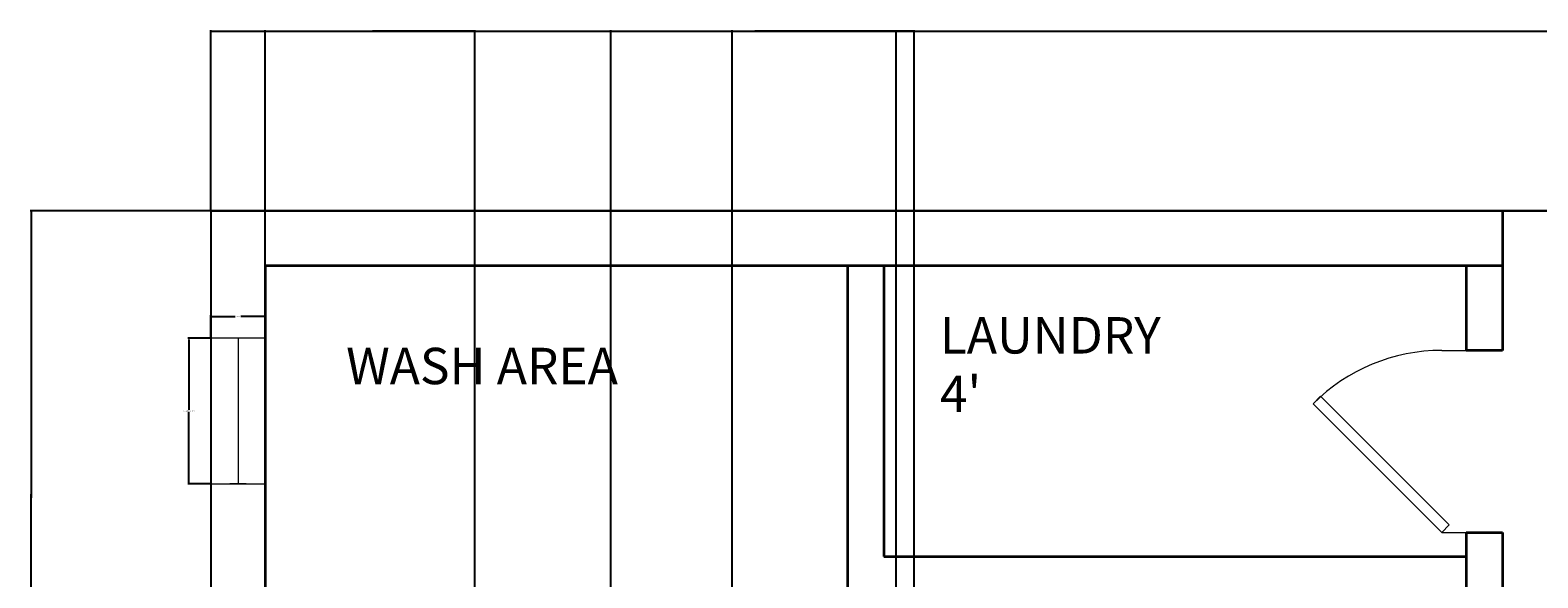
# Model space of a CAD drawing. Units: inches. Extents: x 450 to 1026, y 542 to 1190.
# Tile 9 of 11: x 450 to 698, y 1099 to 1190. Entities that reach past the tile are written whole.
import ezdxf

# ---------------------------------------------------------------- set-up
doc = ezdxf.new("R2010")
doc.units = ezdxf.units.IN
doc.header["$MEASUREMENT"] = 0
for name, color, linetype, lineweight in [('A-ANNO-DIMS', 2, 'Continuous', 18), ('A-AREA-IDEN', 7, 'Continuous', 18), ('A-DOOR', 4, 'Continuous', 18), ('A-GLAZ', 4, 'Continuous', 18), ('A-WALL', 7, 'Continuous', 35), ('C-PROP', 7, 'Continuous', 25)]:
    doc.layers.add(name, color=color, linetype=linetype, lineweight=lineweight)
doc.styles.get("Standard").update_dxf_attribs({"font": 'arial.ttf'})
doc.dimstyles.get("Standard").update_dxf_attribs({"dimtxt": 0.18, "dimasz": 0.18, "dimexe": 0.18, "dimexo": 0.0625, "dimgap": 0.09, "dimtad": 0, "dimtih": 1, "dimtoh": 1, "dimdec": 4, "dimzin": 0, "dimdsep": 46, "dimtxsty": 'Standard', "dimcen": 0.09, "dimadec": 0, "dimazin": 0, "dimtfac": 1, "dimtdec": 4, "dimtofl": 0, "dimtmove": 0, "dimatfit": 3, "dimfxl": 1, "dimtolj": 1, "dimtzin": 0, "dimarcsym": 0})

# ---------------------------------------------------------------- blocks, each defined once
blk = doc.blocks.new('*U4')
for p, q in [((0, 0), (0, -100)), ((750, 0), (750, -100))]:
    blk.add_line(p, q)
blk.add_lwpolyline([(0, 0), (530.3, 530.3), (561.3, 499.4), (30.9, -30.9)], close=True)
blk.add_arc((0, 0), 750, 0, 45)
blk = doc.blocks.new('*U3')
for p, q in [((0, 100), (0, 0)), ((900, 100), (900, 0)), ((0, 50), (900, 50))]:
    blk.add_line(p, q)
blk = doc.blocks.new('WIN-FRAME-24IN')
for p, q in [((9, 24), (0, 24)), ((0, 24), (0, 0)), ((0, 0), (9, 0))]:
    blk.add_line(p, q)
blk = doc.blocks.new('*D37')
at = {"layer": 'A-ANNO-DIMS', "color": 0, "lineweight": -2, "transparency": 16777216}
for p, q in [((479.59, 1138.94), (475.87, 1138.94)), ((476.05, 1138.76), (476.05, 1127.13)), ((476.05, 1115.12), (476.05, 1126.76)), ((479.59, 1114.94), (475.87, 1114.94))]:
    blk.add_line(p, q, dxfattribs=at)
at = {"layer": 'A-ANNO-DIMS', "color": 0, "transparency": 16777216}
for points in [[(476.02, 1138.76), (476.08, 1138.76), (476.05, 1138.94)], [(476.02, 1115.12), (476.08, 1115.12), (476.05, 1114.94)]]:
    blk.add_solid(points, dxfattribs=at)
at = {"layer": 'Defpoints', "color": 0, "transparency": 16777216}
for p in [(476.05, 1138.94), (479.65, 1138.94), (479.65, 1114.94)]:
    blk.add_point(p, dxfattribs=at)
at = {"layer": 'A-ANNO-DIMS', "color": 0, "transparency": 16777216, "insert": (476.05, 1126.94), "char_height": 0.18, "attachment_point": 5}
blk.add_mtext('\\A1;WINDOW 24 TYP.', dxfattribs=at)
blk = doc.blocks.new('*D38')
at = {"layer": 'A-ANNO-DIMS', "color": 0, "lineweight": -2, "transparency": 16777216}
for p, q in [((479.65, 1139.01), (479.65, 1142.72)), ((479.83, 1142.54), (483.69, 1142.54)), ((488.47, 1142.54), (484.61, 1142.54)), ((488.65, 1139.01), (488.65, 1142.72))]:
    blk.add_line(p, q, dxfattribs=at)
at = {"layer": 'A-ANNO-DIMS', "color": 0, "transparency": 16777216}
for points in [[(479.83, 1142.57), (479.83, 1142.51), (479.65, 1142.54)], [(488.47, 1142.57), (488.47, 1142.51), (488.65, 1142.54)]]:
    blk.add_solid(points, dxfattribs=at)
at = {"layer": 'Defpoints', "color": 0, "transparency": 16777216}
for p in [(488.65, 1142.54), (479.65, 1138.94), (488.65, 1138.94)]:
    blk.add_point(p, dxfattribs=at)
at = {"layer": 'A-ANNO-DIMS', "color": 0, "transparency": 16777216, "insert": (484.15, 1142.54), "char_height": 0.18, "attachment_point": 5}
blk.add_mtext('\\A1;9 TYP.', dxfattribs=at)
blk = doc.blocks.new('*D47')
at = {"layer": 'A-ANNO-DIMS', "color": 0, "lineweight": -2, "transparency": 16777216}
for p, q in [((479.65, 1160.01), (479.65, 1189.72)), ((479.83, 1189.54), (719.36, 1189.54)), ((959.47, 1189.54), (719.94, 1189.54)), ((959.65, 1065.01), (959.65, 1189.72))]:
    blk.add_line(p, q, dxfattribs=at)
at = {"layer": 'A-ANNO-DIMS', "color": 0, "transparency": 16777216}
for points in [[(479.83, 1189.57), (479.83, 1189.51), (479.65, 1189.54)], [(959.47, 1189.57), (959.47, 1189.51), (959.65, 1189.54)]]:
    blk.add_solid(points, dxfattribs=at)
at = {"layer": 'Defpoints', "color": 0, "transparency": 16777216}
for p in [(959.65, 1189.54), (479.65, 1159.94), (959.65, 1064.94)]:
    blk.add_point(p, dxfattribs=at)
at = {"layer": 'A-ANNO-DIMS', "color": 0, "transparency": 16777216, "insert": (719.65, 1189.54), "char_height": 0.18, "attachment_point": 5}
blk.add_mtext('\\A1;480', dxfattribs=at)
blk = doc.blocks.new('*D49')
at = {"layer": 'A-ANNO-DIMS', "color": 0, "lineweight": -2, "transparency": 16777216}
for p, q in [((479.59, 1159.94), (449.87, 1159.94)), ((450.05, 1159.76), (450.05, 1113.62)), ((450.05, 1067.12), (450.05, 1113.26)), ((479.59, 1066.94), (449.87, 1066.94))]:
    blk.add_line(p, q, dxfattribs=at)
at = {"layer": 'A-ANNO-DIMS', "color": 0, "transparency": 16777216}
for points in [[(450.02, 1159.76), (450.08, 1159.76), (450.05, 1159.94)], [(450.02, 1067.12), (450.08, 1067.12), (450.05, 1066.94)]]:
    blk.add_solid(points, dxfattribs=at)
at = {"layer": 'Defpoints', "color": 0, "transparency": 16777216}
for p in [(479.65, 1159.94), (450.05, 1066.94), (479.65, 1066.94)]:
    blk.add_point(p, dxfattribs=at)
at = {"layer": 'A-ANNO-DIMS', "color": 0, "transparency": 16777216, "insert": (450.05, 1113.44), "char_height": 0.18, "attachment_point": 5}
blk.add_mtext('\\A1;93', dxfattribs=at)
blk = doc.blocks.new('*D55')
at = {"layer": 'A-ANNO-DIMS', "color": 0, "lineweight": -2, "transparency": 16777216}
for p, q in [((995.59, 1159.94), (449.87, 1159.94)), ((450.05, 1159.76), (450.05, 1112.62)), ((450.05, 1065.12), (450.05, 1112.26)), ((959.59, 1064.94), (449.87, 1064.94))]:
    blk.add_line(p, q, dxfattribs=at)
at = {"layer": 'A-ANNO-DIMS', "color": 0, "transparency": 16777216}
for points in [[(450.02, 1159.76), (450.08, 1159.76), (450.05, 1159.94)], [(450.02, 1065.12), (450.08, 1065.12), (450.05, 1064.94)]]:
    blk.add_solid(points, dxfattribs=at)
at = {"layer": 'Defpoints', "color": 0, "transparency": 16777216}
for p in [(995.65, 1159.94), (450.05, 1064.94), (959.65, 1064.94)]:
    blk.add_point(p, dxfattribs=at)
at = {"layer": 'A-ANNO-DIMS', "color": 0, "transparency": 16777216, "insert": (450.05, 1112.44), "char_height": 0.18, "attachment_point": 5}
blk.add_mtext('\\A1;95', dxfattribs=at)
blk = doc.blocks.new('*D56')
at = {"layer": 'A-ANNO-DIMS', "color": 0, "lineweight": -2, "transparency": 16777216}
for p, q in [((488.65, 1150.88), (488.65, 542.16)), ((584.65, 1150.88), (584.65, 542.16)), ((488.83, 542.34), (536.43, 542.34)), ((584.47, 542.34), (536.87, 542.34))]:
    blk.add_line(p, q, dxfattribs=at)
at = {"layer": 'A-ANNO-DIMS', "color": 0, "transparency": 16777216}
for points in [[(488.83, 542.37), (488.83, 542.31), (488.65, 542.34)], [(584.47, 542.37), (584.47, 542.31), (584.65, 542.34)]]:
    blk.add_solid(points, dxfattribs=at)
at = {"layer": 'Defpoints', "color": 0, "transparency": 16777216}
for p in [(488.65, 1150.94), (584.65, 1150.94), (584.65, 542.34)]:
    blk.add_point(p, dxfattribs=at)
at = {"layer": 'A-ANNO-DIMS', "color": 0, "transparency": 16777216, "insert": (536.65, 542.34), "char_height": 0.18, "attachment_point": 5}
blk.add_mtext('\\A1;96', dxfattribs=at)
blk = doc.blocks.new('*D58')
at = {"layer": 'A-ANNO-DIMS', "color": 0, "lineweight": -2, "transparency": 16777216}
for p, q in [((545.65, 971.01), (545.65, 1189.72)), ((545.83, 1189.54), (568.93, 1189.54)), ((592.47, 1189.54), (569.37, 1189.54)), ((592.65, 977.01), (592.65, 1189.72))]:
    blk.add_line(p, q, dxfattribs=at)
at = {"layer": 'A-ANNO-DIMS', "color": 0, "transparency": 16777216}
for points in [[(545.83, 1189.57), (545.83, 1189.51), (545.65, 1189.54)], [(592.47, 1189.57), (592.47, 1189.51), (592.65, 1189.54)]]:
    blk.add_solid(points, dxfattribs=at)
at = {"layer": 'Defpoints', "color": 0, "transparency": 16777216}
for p in [(592.65, 1189.54), (592.65, 976.94), (545.65, 970.94)]:
    blk.add_point(p, dxfattribs=at)
at = {"layer": 'A-ANNO-DIMS', "color": 0, "transparency": 16777216, "insert": (569.15, 1189.54), "char_height": 0.18, "attachment_point": 5}
blk.add_mtext('\\A1;47', dxfattribs=at)
blk = doc.blocks.new('*D67')
at = {"layer": 'A-ANNO-DIMS', "color": 0, "lineweight": -2, "transparency": 16777216}
for p, q in [((488.65, 1029.39), (488.65, 1189.72)), ((488.83, 1189.54), (505.54, 1189.54)), ((523.04, 1189.54), (506.33, 1189.54)), ((523.22, 1029.39), (523.22, 1189.72))]:
    blk.add_line(p, q, dxfattribs=at)
at = {"layer": 'A-ANNO-DIMS', "color": 0, "transparency": 16777216}
for points in [[(488.83, 1189.57), (488.83, 1189.51), (488.65, 1189.54)], [(523.04, 1189.57), (523.04, 1189.51), (523.22, 1189.54)]]:
    blk.add_solid(points, dxfattribs=at)
at = {"layer": 'Defpoints', "color": 0, "transparency": 16777216}
for p in [(523.22, 1189.54), (488.65, 1029.33), (523.22, 1029.33)]:
    blk.add_point(p, dxfattribs=at)
at = {"layer": 'A-ANNO-DIMS', "color": 0, "transparency": 16777216, "insert": (505.94, 1189.54), "char_height": 0.18, "attachment_point": 5}
blk.add_mtext('\\A1;34.57', dxfattribs=at)
blk = doc.blocks.new('*D70')
at = {"layer": 'A-ANNO-DIMS', "color": 0, "lineweight": -2, "transparency": 16777216}
for p, q in [((565.65, 713.01), (565.65, 1189.72)), ((565.83, 1189.54), (580.43, 1189.54)), ((595.47, 1189.54), (580.87, 1189.54)), ((595.65, 713.01), (595.65, 1189.72))]:
    blk.add_line(p, q, dxfattribs=at)
at = {"layer": 'A-ANNO-DIMS', "color": 0, "transparency": 16777216}
for points in [[(565.83, 1189.57), (565.83, 1189.51), (565.65, 1189.54)], [(595.47, 1189.57), (595.47, 1189.51), (595.65, 1189.54)]]:
    blk.add_solid(points, dxfattribs=at)
at = {"layer": 'Defpoints', "color": 0, "transparency": 16777216}
for p in [(595.65, 1189.54), (565.65, 712.94), (595.65, 712.94)]:
    blk.add_point(p, dxfattribs=at)
at = {"layer": 'A-ANNO-DIMS', "color": 0, "transparency": 16777216, "insert": (580.65, 1189.54), "char_height": 0.18, "attachment_point": 5}
blk.add_mtext('\\A1;30', dxfattribs=at)

msp = doc.modelspace()

# ---------------------------------------------------------------- linework, layer by layer
at = {"layer": 'A-WALL'}
for p, q in [((692.6513, 1159.9426), (692.6513, 1136.9426)), ((488.6513, 1150.9426), (488.6513, 970.9426)), ((488.6513, 1150.9426), (692.6513, 1150.9426)), ((584.6513, 1150.9426), (584.6513, 1096.9426)), ((590.6513, 1150.9426), (590.6513, 1102.9426)), ((686.6513, 1150.9426), (686.6513, 1136.9426)), ((692.6513, 1136.9426), (686.6513, 1136.9426)), ((686.6513, 1106.9426), (692.6513, 1106.9426)), ((686.6513, 1106.9426), (686.6513, 1014.9426)), ((692.6513, 1106.9426), (692.6513, 1014.9426)), ((590.6513, 1102.9426), (686.6513, 1102.9426))]:
    msp.add_line(p, q, dxfattribs=at)
at = {"layer": 'C-PROP'}
for q in [(995.6513, 1159.9426), (479.6513, 571.9426)]:
    msp.add_line((479.6513, 1159.9426), q, dxfattribs=at)

# ---------------------------------------------------------------- block references
at = {"layer": 'A-DOOR', "xscale": 0.04, "yscale": 0.04, "zscale": 0.04, "rotation": 90}
msp.add_blockref('*U4', (682.6513, 1106.9426), dxfattribs=at)
at = {"layer": 'A-GLAZ'}
msp.add_blockref('WIN-FRAME-24IN', (479.651, 1114.943), dxfattribs=at)
at = {"layer": 'A-GLAZ', "xscale": 0.0266666666666667, "yscale": 0.0266666666666667, "zscale": 0.0266666666666667, "rotation": 270}
msp.add_blockref('*U3', (482.818, 1138.9426), dxfattribs=at)

# ---------------------------------------------------------------- texts
at = {"layer": 'A-AREA-IDEN'}
for s, p in [('LAUNDRY', (599.8841, 1136.4223)), ('WASH AREA  ', (501.981, 1131.3672)), ("4'", (599.8841, 1126.7838))]:
    msp.add_text(s, height=6, dxfattribs=at).set_placement(p)

# ---------------------------------------------------------------- dimensions: what is measured, and where the dimension line sits
at = {"layer": 'A-ANNO-DIMS'}
for base, p1, p2, override, picture, middle in [((959.6513, 1189.5426), (479.6513, 1159.9426), (959.6513, 1064.9426), {"dimdec": 0, "dimlfac": 1, "dimrnd": 0, "dimzin": 0, "dimdsep": 46, "dimlunit": 2}, '*D47', (719.6513, 1189.5426)), ((523.2237, 1189.5426), (488.6513, 1029.3314), (523.2237, 1029.3314), {"dimdec": 2, "dimlfac": 1, "dimrnd": 0, "dimzin": 0, "dimdsep": 46, "dimlunit": 2}, '*D67', (505.9375, 1189.5426)), ((592.6513, 1189.5426), (545.6513, 970.9426), (592.6513, 976.9426), {"dimdec": 0, "dimlfac": 1, "dimrnd": 0, "dimzin": 0, "dimdsep": 46, "dimlunit": 2}, '*D58', (569.1513, 1189.5426)), ((595.6513, 1189.5426), (565.6513, 712.9426), (595.6513, 712.9426), {"dimdec": 0, "dimlfac": 1, "dimrnd": 0, "dimzin": 0, "dimdsep": 46, "dimlunit": 2}, '*D70', (580.6513, 1189.5426)), ((584.6513, 542.3426), (488.6513, 1150.9426), (584.6513, 1150.9426), {"dimdec": 0, "dimlfac": 1, "dimrnd": 0, "dimzin": 0, "dimdsep": 46, "dimlunit": 2}, '*D56', (536.6513, 542.3426))]:
    dim = msp.add_linear_dim(base=base, p1=p1, p2=p2, dimstyle='Standard', override=override, dxfattribs=at)
    dim.commit()
    dim.dimension.update_dxf_attribs({"geometry": picture, "text_midpoint": middle})
for base, p1, p2, picture, middle in [((450.0513, 1066.9426), (479.6513, 1159.9426), (479.6513, 1066.9426), '*D49', (450.0513, 1113.4426)), ((450.0513, 1064.9426), (995.6513, 1159.9426), (959.6513, 1064.9426), '*D55', (450.0513, 1112.4426))]:
    dim = msp.add_linear_dim(base=base, p1=p1, p2=p2, angle=90, dimstyle='Standard', override={"dimdec": 0, "dimlfac": 1, "dimrnd": 0, "dimzin": 0, "dimdsep": 46, "dimlunit": 2}, dxfattribs=at)
    dim.commit()
    dim.dimension.update_dxf_attribs({"geometry": picture, "text_midpoint": middle})
dim = msp.add_linear_dim(base=(488.6513, 1142.5426), p1=(479.6513, 1138.9426), p2=(488.6513, 1138.9426), text='<> TYP.', dimstyle='Standard', override={"dimdec": 0, "dimlfac": 1, "dimrnd": 0, "dimzin": 0, "dimdsep": 46, "dimlunit": 2}, dxfattribs=at)
dim.commit()
dim.dimension.update_dxf_attribs({"geometry": '*D38', "text_midpoint": (484.1513, 1142.5426)})
dim = msp.add_linear_dim(base=(476.0513, 1138.9426), p1=(479.6513, 1114.9426), p2=(479.6513, 1138.9426), angle=90, text='WINDOW <> TYP.', dimstyle='Standard', override={"dimdec": 0, "dimlfac": 1, "dimrnd": 0, "dimzin": 0, "dimdsep": 46, "dimlunit": 2}, dxfattribs=at)
dim.commit()
dim.dimension.update_dxf_attribs({"geometry": '*D37', "text_midpoint": (476.0513, 1126.9426)})

doc.saveas('drawing.dxf')
